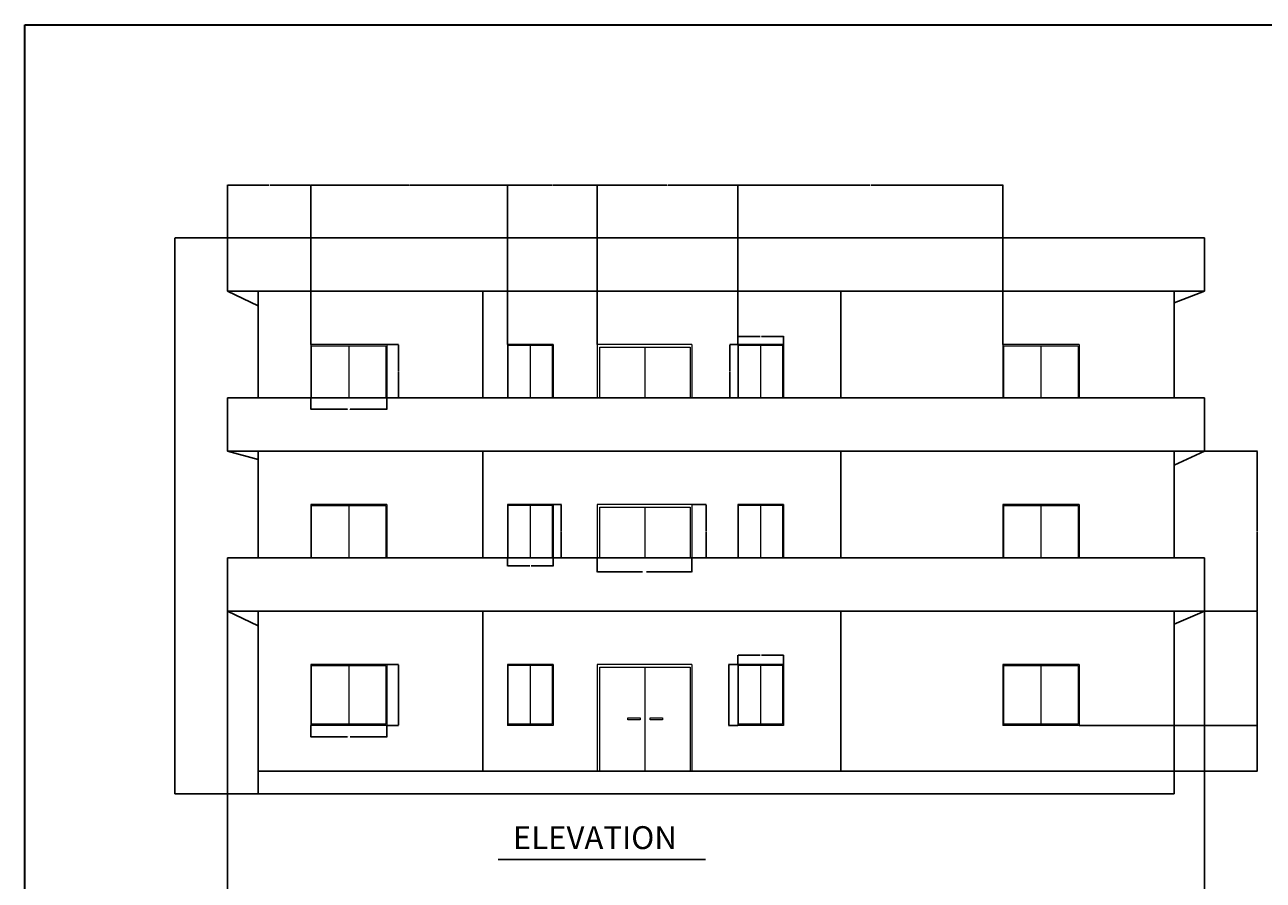
# Model space of a CAD drawing. Units: inches. Extents: x 2185 to 4426, y 1138 to 3073.
# Tile 7 of 14: x 2185 to 3160, y 2400 to 3073. Entities that reach past the tile are written whole.
import ezdxf

# ---------------------------------------------------------------- set-up
doc = ezdxf.new("R2010")
doc.units = ezdxf.units.IN
for name, color, linetype, lineweight in [('A-ANNO-DIMS', 2, 'Continuous', 18), ('A-ANNO-TITL', 7, 'Continuous', 25), ('A-ANNO-TTLB', 7, 'Continuous', 35), ('A-ELEV', 7, 'Continuous', 25), ('A-ELEV-DOOR', 3, 'Continuous', 18), ('A-ELEV-GLAZ', 4, 'Continuous', 18)]:
    doc.layers.add(name, color=color, linetype=linetype, lineweight=lineweight)
doc.styles.get("Standard").update_dxf_attribs({"font": 'arial.ttf'})
doc.dimstyles.get("Standard").update_dxf_attribs({"dimtxt": 0.18, "dimasz": 0.18, "dimexe": 0.18, "dimexo": 0.0625, "dimgap": 0.09, "dimtad": 0, "dimtih": 1, "dimtoh": 1, "dimdec": 4, "dimzin": 0, "dimdsep": 46, "dimtxsty": 'Standard', "dimcen": 0.09, "dimadec": 0, "dimazin": 0, "dimtfac": 1, "dimtdec": 4, "dimtofl": 0, "dimtmove": 0, "dimatfit": 3, "dimfxl": 1, "dimtolj": 1, "dimtzin": 0, "dimarcsym": 0})

# ---------------------------------------------------------------- blocks, each defined once
blk = doc.blocks.new('WIN-ELEV-WIDE-LOWER')
for p, q in [((0, 48), (0, 0)), ((60, 48), (0, 48)), ((0, 48), (0, 0)), ((60, 48), (0, 48)), ((29.88, 47.09), (29.88, 0.99)), ((60, 48), (60, 0)), ((60, 48), (60, 0)), ((60, 0), (0, 0)), ((60, 0), (0, 0))]:
    blk.add_line(p, q)
blk.add_lwpolyline([(0.58, 47.09), (59.17, 47.09), (59.17, 0.99), (0.58, 0.99)], close=True)
blk = doc.blocks.new('WIN-ELEV-WIDE-UPPER')
for p, q in [((0, 42), (0, 0)), ((60, 42), (0, 42)), ((0, 42), (0, 0)), ((60, 42), (0, 42)), ((29.88, 41.09), (29.88, 0)), ((60, 42), (60, 0)), ((60, 42), (60, 0))]:
    blk.add_line(p, q)
blk.add_lwpolyline([(0.58, 0), (0.58, 41.09), (59.17, 41.09), (59.17, 0)])
blk = doc.blocks.new('WIN-ELEV-NARROW-UPPER')
for p, q in [((0, 42), (0, 0)), ((36, 42), (0, 42)), ((0, 42), (0, 0)), ((36, 42), (0, 42)), ((0, 42), (0, 0)), ((17.83, 41.41), (17.83, 0)), ((36, 42), (36, 0)), ((36, 42), (36, 0)), ((36, 42), (36, 0))]:
    blk.add_line(p, q)
blk.add_lwpolyline([(0.51, 0), (0.51, 41.41), (35.15, 41.41), (35.15, 0)])
blk = doc.blocks.new('WIN-ELEV-NARROW-LOWER-TYPE-B')
for p, q in [((0, 48), (0, 0)), ((36, 48), (0, 48)), ((17.83, 47.41), (17.83, 0.85)), ((36, 48), (36, 0)), ((36, 0), (0, 0))]:
    blk.add_line(p, q)
blk.add_lwpolyline([(0.51, 47.41), (35.15, 47.41), (35.15, 0.85), (0.51, 0.85)], close=True)
blk = doc.blocks.new('WIN-ELEV-NARROW-UPPER-TYPE-B')
for p, q in [((0, 42), (0, 0)), ((36, 42), (0, 42)), ((17.83, 41.41), (17.83, 0)), ((36, 42), (36, 0))]:
    blk.add_line(p, q)
blk.add_lwpolyline([(0.51, 0), (0.51, 41.41), (35.15, 41.41), (35.15, 0)])
blk = doc.blocks.new('DOOR-ELEV-DOUBLE-UPPER-TYPE-B')
for p, q in [((0, 42), (0, 0)), ((74.51, 42), (0, 42)), ((37.6, 39.93), (37.6, 0)), ((74.51, 42), (74.51, 0))]:
    blk.add_line(p, q)
blk.add_lwpolyline([(2.14, 0), (2.14, 39.93), (73.06, 39.93), (73.06, 0)])
blk = doc.blocks.new('*D126')
at = {"layer": 'A-ANNO-DIMS', "color": 0, "lineweight": -2, "transparency": 16777216}
for p, q in [((2410.04, 2521.42), (2410.04, 2512.3)), ((2470.04, 2521.42), (2470.04, 2512.3)), ((2410.22, 2512.48), (2438.92, 2512.48)), ((2469.86, 2512.48), (2441.16, 2512.48))]:
    blk.add_line(p, q, dxfattribs=at)
at = {"layer": 'A-ANNO-DIMS', "color": 0, "transparency": 16777216}
for points in [[(2410.22, 2512.51), (2410.22, 2512.45), (2410.04, 2512.48)], [(2469.86, 2512.51), (2469.86, 2512.45), (2470.04, 2512.48)]]:
    blk.add_solid(points, dxfattribs=at)
at = {"layer": 'Defpoints', "color": 0, "transparency": 16777216}
for p in [(2410.04, 2521.48), (2470.04, 2521.48), (2470.04, 2512.48)]:
    blk.add_point(p, dxfattribs=at)
at = {"layer": 'A-ANNO-DIMS', "color": 0, "transparency": 16777216, "insert": (2440.04, 2512.48), "char_height": 0.18, "attachment_point": 5}
blk.add_mtext('\\A1;WINDOW 60 TYP.', dxfattribs=at)
blk = doc.blocks.new('*D127')
at = {"layer": 'A-ANNO-DIMS', "color": 0, "lineweight": -2, "transparency": 16777216}
for p, q in [((2470.1, 2569.48), (2479.22, 2569.48)), ((2479.04, 2569.3), (2479.04, 2545.66)), ((2479.04, 2521.66), (2479.04, 2545.3)), ((2470.1, 2521.48), (2479.22, 2521.48))]:
    blk.add_line(p, q, dxfattribs=at)
at = {"layer": 'A-ANNO-DIMS', "color": 0, "transparency": 16777216}
for points in [[(2479.01, 2569.3), (2479.07, 2569.3), (2479.04, 2569.48)], [(2479.01, 2521.66), (2479.07, 2521.66), (2479.04, 2521.48)]]:
    blk.add_solid(points, dxfattribs=at)
at = {"layer": 'Defpoints', "color": 0, "transparency": 16777216}
for p in [(2470.04, 2569.48), (2479.04, 2569.48), (2470.04, 2521.48)]:
    blk.add_point(p, dxfattribs=at)
at = {"layer": 'A-ANNO-DIMS', "color": 0, "transparency": 16777216, "insert": (2479.04, 2545.48), "char_height": 0.18, "attachment_point": 5}
blk.add_mtext('\\A1;48 TYP.', dxfattribs=at)
blk = doc.blocks.new('*D128')
at = {"layer": 'A-ANNO-DIMS', "color": 0, "lineweight": -2, "transparency": 16777216}
for p, q in [((2410.04, 2779.42), (2410.04, 2770.3)), ((2410.22, 2770.48), (2438.92, 2770.48)), ((2469.86, 2770.48), (2441.16, 2770.48)), ((2470.04, 2779.42), (2470.04, 2770.3))]:
    blk.add_line(p, q, dxfattribs=at)
at = {"layer": 'A-ANNO-DIMS', "color": 0, "transparency": 16777216}
for points in [[(2410.22, 2770.51), (2410.22, 2770.45), (2410.04, 2770.48)], [(2469.86, 2770.51), (2469.86, 2770.45), (2470.04, 2770.48)]]:
    blk.add_solid(points, dxfattribs=at)
at = {"layer": 'Defpoints', "color": 0, "transparency": 16777216}
for p in [(2410.04, 2779.48), (2470.04, 2779.48), (2470.04, 2770.48)]:
    blk.add_point(p, dxfattribs=at)
at = {"layer": 'A-ANNO-DIMS', "color": 0, "transparency": 16777216, "insert": (2440.04, 2770.48), "char_height": 0.18, "attachment_point": 5}
blk.add_mtext('\\A1;WINDOW 60 TYP.', dxfattribs=at)
blk = doc.blocks.new('*D129')
at = {"layer": 'A-ANNO-DIMS', "color": 0, "lineweight": -2, "transparency": 16777216}
for p, q in [((2470.1, 2821.48), (2479.22, 2821.48)), ((2479.04, 2821.3), (2479.04, 2800.66)), ((2479.04, 2779.66), (2479.04, 2800.3)), ((2470.1, 2779.48), (2479.22, 2779.48))]:
    blk.add_line(p, q, dxfattribs=at)
at = {"layer": 'A-ANNO-DIMS', "color": 0, "transparency": 16777216}
for points in [[(2479.01, 2821.3), (2479.07, 2821.3), (2479.04, 2821.48)], [(2479.01, 2779.66), (2479.07, 2779.66), (2479.04, 2779.48)]]:
    blk.add_solid(points, dxfattribs=at)
at = {"layer": 'Defpoints', "color": 0, "transparency": 16777216}
for p in [(2470.04, 2821.48), (2479.04, 2821.48), (2470.04, 2779.48)]:
    blk.add_point(p, dxfattribs=at)
at = {"layer": 'A-ANNO-DIMS', "color": 0, "transparency": 16777216, "insert": (2479.04, 2800.48), "char_height": 0.18, "attachment_point": 5}
blk.add_mtext('\\A1;42 TYP.', dxfattribs=at)
blk = doc.blocks.new('*D130')
at = {"layer": 'A-ANNO-DIMS', "color": 0, "lineweight": -2, "transparency": 16777216}
for p, q in [((2601.1, 2695.48), (2607.52, 2695.48)), ((2607.34, 2695.3), (2607.34, 2674.67)), ((2607.34, 2653.66), (2607.34, 2674.3)), ((2601.1, 2653.48), (2607.52, 2653.48))]:
    blk.add_line(p, q, dxfattribs=at)
at = {"layer": 'A-ANNO-DIMS', "color": 0, "transparency": 16777216}
for points in [[(2607.31, 2695.3), (2607.37, 2695.3), (2607.34, 2695.48)], [(2607.31, 2653.66), (2607.37, 2653.66), (2607.34, 2653.48)]]:
    blk.add_solid(points, dxfattribs=at)
at = {"layer": 'Defpoints', "color": 0, "transparency": 16777216}
for p in [(2601.04, 2695.48), (2607.34, 2695.48), (2601.04, 2653.48)]:
    blk.add_point(p, dxfattribs=at)
at = {"layer": 'A-ANNO-DIMS', "color": 0, "transparency": 16777216, "insert": (2607.34, 2674.48), "char_height": 0.18, "attachment_point": 5}
blk.add_mtext('\\A1;SASH 42 TYP.', dxfattribs=at)
blk = doc.blocks.new('*D131')
at = {"layer": 'A-ANNO-DIMS', "color": 0, "lineweight": -2, "transparency": 16777216}
for p, q in [((2565.04, 2653.42), (2565.04, 2647)), ((2601.04, 2653.42), (2601.04, 2647)), ((2565.22, 2647.18), (2582.51, 2647.18)), ((2600.86, 2647.18), (2583.57, 2647.18))]:
    blk.add_line(p, q, dxfattribs=at)
at = {"layer": 'A-ANNO-DIMS', "color": 0, "transparency": 16777216}
for points in [[(2565.22, 2647.21), (2565.22, 2647.15), (2565.04, 2647.18)], [(2600.86, 2647.21), (2600.86, 2647.15), (2601.04, 2647.18)]]:
    blk.add_solid(points, dxfattribs=at)
at = {"layer": 'Defpoints', "color": 0, "transparency": 16777216}
for p in [(2565.04, 2653.48), (2601.04, 2653.48), (2601.04, 2647.18)]:
    blk.add_point(p, dxfattribs=at)
at = {"layer": 'A-ANNO-DIMS', "color": 0, "transparency": 16777216, "insert": (2583.04, 2647.18), "char_height": 0.18, "attachment_point": 5}
blk.add_mtext('\\A1;36 TYP.', dxfattribs=at)
blk = doc.blocks.new('*D132')
at = {"layer": 'A-ANNO-DIMS', "color": 0, "lineweight": -2, "transparency": 16777216}
for p, q in [((2746.37, 2569.48), (2739.05, 2569.48)), ((2739.23, 2569.3), (2739.23, 2545.67)), ((2739.23, 2521.66), (2739.23, 2545.3)), ((2746.37, 2521.48), (2739.05, 2521.48))]:
    blk.add_line(p, q, dxfattribs=at)
at = {"layer": 'A-ANNO-DIMS', "color": 0, "transparency": 16777216}
for points in [[(2739.2, 2569.3), (2739.26, 2569.3), (2739.23, 2569.48)], [(2739.2, 2521.66), (2739.26, 2521.66), (2739.23, 2521.48)]]:
    blk.add_solid(points, dxfattribs=at)
at = {"layer": 'Defpoints', "color": 0, "transparency": 16777216}
for p in [(2739.23, 2569.48), (2746.43, 2569.48), (2746.43, 2521.48)]:
    blk.add_point(p, dxfattribs=at)
at = {"layer": 'A-ANNO-DIMS', "color": 0, "transparency": 16777216, "insert": (2739.23, 2545.48), "char_height": 0.18, "attachment_point": 5}
blk.add_mtext('\\A1;SASH 48 TYP.', dxfattribs=at)
blk = doc.blocks.new('*D133')
at = {"layer": 'A-ANNO-DIMS', "color": 0, "lineweight": -2, "transparency": 16777216}
for p, q in [((2746.43, 2569.54), (2746.43, 2576.86)), ((2746.61, 2576.68), (2763.9, 2576.68)), ((2782.25, 2576.68), (2764.96, 2576.68)), ((2782.43, 2569.54), (2782.43, 2576.86))]:
    blk.add_line(p, q, dxfattribs=at)
at = {"layer": 'A-ANNO-DIMS', "color": 0, "transparency": 16777216}
for points in [[(2746.61, 2576.71), (2746.61, 2576.65), (2746.43, 2576.68)], [(2782.25, 2576.71), (2782.25, 2576.65), (2782.43, 2576.68)]]:
    blk.add_solid(points, dxfattribs=at)
at = {"layer": 'Defpoints', "color": 0, "transparency": 16777216}
for p in [(2782.43, 2576.68), (2746.43, 2569.48), (2782.43, 2569.48)]:
    blk.add_point(p, dxfattribs=at)
at = {"layer": 'A-ANNO-DIMS', "color": 0, "transparency": 16777216, "insert": (2764.43, 2576.68), "char_height": 0.18, "attachment_point": 5}
blk.add_mtext('\\A1;36 TYP.', dxfattribs=at)
blk = doc.blocks.new('*D134')
at = {"layer": 'A-ANNO-DIMS', "color": 0, "lineweight": -2, "transparency": 16777216}
for p, q in [((2746.37, 2821.48), (2739.95, 2821.48)), ((2740.13, 2821.3), (2740.13, 2800.67)), ((2740.13, 2779.66), (2740.13, 2800.3)), ((2746.37, 2779.48), (2739.95, 2779.48))]:
    blk.add_line(p, q, dxfattribs=at)
at = {"layer": 'A-ANNO-DIMS', "color": 0, "transparency": 16777216}
for points in [[(2740.1, 2821.3), (2740.16, 2821.3), (2740.13, 2821.48)], [(2740.1, 2779.66), (2740.16, 2779.66), (2740.13, 2779.48)]]:
    blk.add_solid(points, dxfattribs=at)
at = {"layer": 'Defpoints', "color": 0, "transparency": 16777216}
for p in [(2740.13, 2821.48), (2746.43, 2821.48), (2746.43, 2779.48)]:
    blk.add_point(p, dxfattribs=at)
at = {"layer": 'A-ANNO-DIMS', "color": 0, "transparency": 16777216, "insert": (2740.13, 2800.48), "char_height": 0.18, "attachment_point": 5}
blk.add_mtext('\\A1;SASH 42 TYP.', dxfattribs=at)
blk = doc.blocks.new('*D135')
at = {"layer": 'A-ANNO-DIMS', "color": 0, "lineweight": -2, "transparency": 16777216}
for p, q in [((2746.43, 2821.54), (2746.43, 2827.96)), ((2746.61, 2827.78), (2763.9, 2827.78)), ((2782.25, 2827.78), (2764.96, 2827.78)), ((2782.43, 2821.54), (2782.43, 2827.96))]:
    blk.add_line(p, q, dxfattribs=at)
at = {"layer": 'A-ANNO-DIMS', "color": 0, "transparency": 16777216}
for points in [[(2746.61, 2827.81), (2746.61, 2827.75), (2746.43, 2827.78)], [(2782.25, 2827.81), (2782.25, 2827.75), (2782.43, 2827.78)]]:
    blk.add_solid(points, dxfattribs=at)
at = {"layer": 'Defpoints', "color": 0, "transparency": 16777216}
for p in [(2746.43, 2821.48), (2782.43, 2827.78), (2782.43, 2821.48)]:
    blk.add_point(p, dxfattribs=at)
at = {"layer": 'A-ANNO-DIMS', "color": 0, "transparency": 16777216, "insert": (2764.43, 2827.78), "char_height": 0.18, "attachment_point": 5}
blk.add_mtext('\\A1;36 TYP.', dxfattribs=at)
blk = doc.blocks.new('*D136')
at = {"layer": 'A-ANNO-DIMS', "color": 0, "lineweight": -2, "transparency": 16777216}
for p, q in [((2635.64, 2653.42), (2635.64, 2642.13)), ((2710.16, 2653.42), (2710.16, 2642.13)), ((2635.82, 2642.31), (2671.38, 2642.31)), ((2709.98, 2642.31), (2674.42, 2642.31))]:
    blk.add_line(p, q, dxfattribs=at)
at = {"layer": 'A-ANNO-DIMS', "color": 0, "transparency": 16777216}
for points in [[(2635.82, 2642.34), (2635.82, 2642.28), (2635.64, 2642.31)], [(2709.98, 2642.34), (2709.98, 2642.28), (2710.16, 2642.31)]]:
    blk.add_solid(points, dxfattribs=at)
at = {"layer": 'Defpoints', "color": 0, "transparency": 16777216}
for p in [(2635.64, 2653.48), (2710.16, 2653.48), (2710.16, 2642.31)]:
    blk.add_point(p, dxfattribs=at)
at = {"layer": 'A-ANNO-DIMS', "color": 0, "transparency": 16777216, "insert": (2672.9, 2642.31), "char_height": 0.18, "attachment_point": 5}
blk.add_mtext('\\A1;PAIRED DOORS 75 TYP.', dxfattribs=at)
blk = doc.blocks.new('*D137')
at = {"layer": 'A-ANNO-DIMS', "color": 0, "lineweight": -2, "transparency": 16777216}
for p, q in [((2710.22, 2695.48), (2721.51, 2695.48)), ((2721.33, 2695.3), (2721.33, 2674.66)), ((2721.33, 2653.66), (2721.33, 2674.3)), ((2710.22, 2653.48), (2721.51, 2653.48))]:
    blk.add_line(p, q, dxfattribs=at)
at = {"layer": 'A-ANNO-DIMS', "color": 0, "transparency": 16777216}
for points in [[(2721.3, 2695.3), (2721.36, 2695.3), (2721.33, 2695.48)], [(2721.3, 2653.66), (2721.36, 2653.66), (2721.33, 2653.48)]]:
    blk.add_solid(points, dxfattribs=at)
at = {"layer": 'Defpoints', "color": 0, "transparency": 16777216}
for p in [(2710.16, 2695.48), (2721.33, 2695.48), (2710.16, 2653.48)]:
    blk.add_point(p, dxfattribs=at)
at = {"layer": 'A-ANNO-DIMS', "color": 0, "transparency": 16777216, "insert": (2721.33, 2674.48), "char_height": 0.18, "attachment_point": 5}
blk.add_mtext('\\A1;42 TYP.', dxfattribs=at)
blk = doc.blocks.new('*D162')
at = {"layer": 'A-ANNO-DIMS', "color": 0, "lineweight": -2, "transparency": 16777216}
for p, q in [((2344.52, 2611.42), (2344.52, 2374.27)), ((3114.02, 2611.42), (3114.02, 2374.27)), ((2344.7, 2374.45), (2728.88, 2374.45)), ((3113.84, 2374.45), (2729.66, 2374.45))]:
    blk.add_line(p, q, dxfattribs=at)
at = {"layer": 'A-ANNO-DIMS', "color": 0, "transparency": 16777216}
for points in [[(2344.7, 2374.48), (2344.7, 2374.42), (2344.52, 2374.45)], [(3113.84, 2374.48), (3113.84, 2374.42), (3114.02, 2374.45)]]:
    blk.add_solid(points, dxfattribs=at)
at = {"layer": 'Defpoints', "color": 0, "transparency": 16777216}
for p in [(2344.52, 2611.48), (3114.02, 2611.48), (3114.02, 2374.45)]:
    blk.add_point(p, dxfattribs=at)
at = {"layer": 'A-ANNO-DIMS', "color": 0, "transparency": 16777216, "insert": (2729.27, 2374.45), "char_height": 0.18, "attachment_point": 5}
blk.add_mtext('\\A1;769.5', dxfattribs=at)
blk = doc.blocks.new('*D163')
at = {"layer": 'A-ANNO-DIMS', "color": 0, "lineweight": -2, "transparency": 16777216}
for p, q in [((2344.46, 2905.48), (2302.84, 2905.48)), ((2303.02, 2905.3), (2303.02, 2686.66)), ((2303.02, 2467.66), (2303.02, 2686.3)), ((2368.46, 2467.48), (2302.84, 2467.48))]:
    blk.add_line(p, q, dxfattribs=at)
at = {"layer": 'A-ANNO-DIMS', "color": 0, "transparency": 16777216}
for points in [[(2302.99, 2905.3), (2303.05, 2905.3), (2303.02, 2905.48)], [(2302.99, 2467.66), (2303.05, 2467.66), (2303.02, 2467.48)]]:
    blk.add_solid(points, dxfattribs=at)
at = {"layer": 'Defpoints', "color": 0, "transparency": 16777216}
for p in [(2303.02, 2905.48), (2344.52, 2905.48), (2368.52, 2467.48)]:
    blk.add_point(p, dxfattribs=at)
at = {"layer": 'A-ANNO-DIMS', "color": 0, "transparency": 16777216, "insert": (2303.02, 2686.48), "char_height": 0.18, "attachment_point": 5}
blk.add_mtext('\\A1;438', dxfattribs=at)
blk = doc.blocks.new('*D164')
at = {"layer": 'A-ANNO-DIMS', "color": 0, "lineweight": -2, "transparency": 16777216}
for p, q in [((2344.52, 2905.54), (2344.52, 2947.16)), ((2344.7, 2946.98), (2376.89, 2946.98)), ((2409.86, 2946.98), (2377.67, 2946.98)), ((2410.04, 2821.54), (2410.04, 2947.16))]:
    blk.add_line(p, q, dxfattribs=at)
at = {"layer": 'A-ANNO-DIMS', "color": 0, "transparency": 16777216}
for points in [[(2344.7, 2947.01), (2344.7, 2946.95), (2344.52, 2946.98)], [(2409.86, 2947.01), (2409.86, 2946.95), (2410.04, 2946.98)]]:
    blk.add_solid(points, dxfattribs=at)
at = {"layer": 'Defpoints', "color": 0, "transparency": 16777216}
for p in [(2410.04, 2946.98), (2344.52, 2905.48), (2410.04, 2821.48)]:
    blk.add_point(p, dxfattribs=at)
at = {"layer": 'A-ANNO-DIMS', "color": 0, "transparency": 16777216, "insert": (2377.28, 2946.98), "char_height": 0.18, "attachment_point": 5}
blk.add_mtext('\\A1;65.52', dxfattribs=at)
blk = doc.blocks.new('*D165')
at = {"layer": 'A-ANNO-DIMS', "color": 0, "lineweight": -2, "transparency": 16777216}
for p, q in [((2410.04, 2821.54), (2410.04, 2947.16)), ((2410.22, 2946.98), (2487.26, 2946.98)), ((2564.86, 2946.98), (2487.82, 2946.98)), ((2565.04, 2821.54), (2565.04, 2947.16))]:
    blk.add_line(p, q, dxfattribs=at)
at = {"layer": 'A-ANNO-DIMS', "color": 0, "transparency": 16777216}
for points in [[(2410.22, 2947.01), (2410.22, 2946.95), (2410.04, 2946.98)], [(2564.86, 2947.01), (2564.86, 2946.95), (2565.04, 2946.98)]]:
    blk.add_solid(points, dxfattribs=at)
at = {"layer": 'Defpoints', "color": 0, "transparency": 16777216}
for p in [(2565.04, 2946.98), (2410.04, 2821.48), (2565.04, 2821.48)]:
    blk.add_point(p, dxfattribs=at)
at = {"layer": 'A-ANNO-DIMS', "color": 0, "transparency": 16777216, "insert": (2487.54, 2946.98), "char_height": 0.18, "attachment_point": 5}
blk.add_mtext('\\A1;155', dxfattribs=at)
blk = doc.blocks.new('*D166')
at = {"layer": 'A-ANNO-DIMS', "color": 0, "lineweight": -2, "transparency": 16777216}
for p, q in [((2565.04, 2821.54), (2565.04, 2947.16)), ((2565.22, 2946.98), (2600.02, 2946.98)), ((2635.46, 2946.98), (2600.66, 2946.98)), ((2635.64, 2821.54), (2635.64, 2947.16))]:
    blk.add_line(p, q, dxfattribs=at)
at = {"layer": 'A-ANNO-DIMS', "color": 0, "transparency": 16777216}
for points in [[(2565.22, 2947.01), (2565.22, 2946.95), (2565.04, 2946.98)], [(2635.46, 2947.01), (2635.46, 2946.95), (2635.64, 2946.98)]]:
    blk.add_solid(points, dxfattribs=at)
at = {"layer": 'Defpoints', "color": 0, "transparency": 16777216}
for p in [(2635.64, 2946.98), (2565.04, 2821.48), (2635.64, 2821.48)]:
    blk.add_point(p, dxfattribs=at)
at = {"layer": 'A-ANNO-DIMS', "color": 0, "transparency": 16777216, "insert": (2600.34, 2946.98), "char_height": 0.18, "attachment_point": 5}
blk.add_mtext('\\A1;70.6', dxfattribs=at)
blk = doc.blocks.new('*D167')
at = {"layer": 'A-ANNO-DIMS', "color": 0, "lineweight": -2, "transparency": 16777216}
for p, q in [((2635.64, 2821.54), (2635.64, 2947.16)), ((2635.82, 2946.98), (2690.58, 2946.98)), ((2746.25, 2946.98), (2691.49, 2946.98)), ((2746.43, 2821.54), (2746.43, 2947.16))]:
    blk.add_line(p, q, dxfattribs=at)
at = {"layer": 'A-ANNO-DIMS', "color": 0, "transparency": 16777216}
for points in [[(2635.82, 2947.01), (2635.82, 2946.95), (2635.64, 2946.98)], [(2746.25, 2947.01), (2746.25, 2946.95), (2746.43, 2946.98)]]:
    blk.add_solid(points, dxfattribs=at)
at = {"layer": 'Defpoints', "color": 0, "transparency": 16777216}
for p in [(2746.43, 2946.98), (2635.64, 2821.48), (2746.43, 2821.48)]:
    blk.add_point(p, dxfattribs=at)
at = {"layer": 'A-ANNO-DIMS', "color": 0, "transparency": 16777216, "insert": (2691.04, 2946.98), "char_height": 0.18, "attachment_point": 5}
blk.add_mtext('\\A1;110.79', dxfattribs=at)
blk = doc.blocks.new('*D168')
at = {"layer": 'A-ANNO-DIMS', "color": 0, "lineweight": -2, "transparency": 16777216}
for p, q in [((2746.43, 2821.54), (2746.43, 2947.16)), ((2746.61, 2946.98), (2850.43, 2946.98)), ((2955.03, 2946.98), (2851.22, 2946.98)), ((2955.21, 2821.54), (2955.21, 2947.16))]:
    blk.add_line(p, q, dxfattribs=at)
at = {"layer": 'A-ANNO-DIMS', "color": 0, "transparency": 16777216}
for points in [[(2746.61, 2947.01), (2746.61, 2946.95), (2746.43, 2946.98)], [(2955.03, 2947.01), (2955.03, 2946.95), (2955.21, 2946.98)]]:
    blk.add_solid(points, dxfattribs=at)
at = {"layer": 'Defpoints', "color": 0, "transparency": 16777216}
for p in [(2955.21, 2946.98), (2746.43, 2821.48), (2955.21, 2821.48)]:
    blk.add_point(p, dxfattribs=at)
at = {"layer": 'A-ANNO-DIMS', "color": 0, "transparency": 16777216, "insert": (2850.82, 2946.98), "char_height": 0.18, "attachment_point": 5}
blk.add_mtext('\\A1;208.8', dxfattribs=at)
blk = doc.blocks.new('*D169')
at = {"layer": 'A-ANNO-DIMS', "color": 0, "lineweight": -2, "transparency": 16777216}
for p, q in [((3015.27, 2521.48), (3155.7, 2521.48)), ((3155.52, 2521.3), (3155.52, 2503.66)), ((3155.52, 2485.66), (3155.52, 2503.3)), ((3090.08, 2485.48), (3155.7, 2485.48))]:
    blk.add_line(p, q, dxfattribs=at)
at = {"layer": 'A-ANNO-DIMS', "color": 0, "transparency": 16777216}
for points in [[(3155.49, 2521.3), (3155.55, 2521.3), (3155.52, 2521.48)], [(3155.49, 2485.66), (3155.55, 2485.66), (3155.52, 2485.48)]]:
    blk.add_solid(points, dxfattribs=at)
at = {"layer": 'Defpoints', "color": 0, "transparency": 16777216}
for p in [(3015.21, 2521.48), (3155.52, 2521.48), (3090.02, 2485.48)]:
    blk.add_point(p, dxfattribs=at)
at = {"layer": 'A-ANNO-DIMS', "color": 0, "transparency": 16777216, "insert": (3155.52, 2503.48), "char_height": 0.18, "attachment_point": 5}
blk.add_mtext('\\A1;36', dxfattribs=at)
blk = doc.blocks.new('*D170')
at = {"layer": 'A-ANNO-DIMS', "color": 0, "lineweight": -2, "transparency": 16777216}
for p, q in [((3114.08, 2611.48), (3155.7, 2611.48)), ((3155.52, 2611.3), (3155.52, 2566.66)), ((3155.52, 2521.66), (3155.52, 2566.3)), ((3015.27, 2521.48), (3155.7, 2521.48))]:
    blk.add_line(p, q, dxfattribs=at)
at = {"layer": 'A-ANNO-DIMS', "color": 0, "transparency": 16777216}
for points in [[(3155.49, 2611.3), (3155.55, 2611.3), (3155.52, 2611.48)], [(3155.49, 2521.66), (3155.55, 2521.66), (3155.52, 2521.48)]]:
    blk.add_solid(points, dxfattribs=at)
at = {"layer": 'Defpoints', "color": 0, "transparency": 16777216}
for p in [(3114.02, 2611.48), (3155.52, 2611.48), (3015.21, 2521.48)]:
    blk.add_point(p, dxfattribs=at)
at = {"layer": 'A-ANNO-DIMS', "color": 0, "transparency": 16777216, "insert": (3155.52, 2566.48), "char_height": 0.18, "attachment_point": 5}
blk.add_mtext('\\A1;90', dxfattribs=at)
blk = doc.blocks.new('*D171')
at = {"layer": 'A-ANNO-DIMS', "color": 0, "lineweight": -2, "transparency": 16777216}
for p, q in [((3114.08, 2737.48), (3155.7, 2737.48)), ((3155.52, 2737.3), (3155.52, 2674.66)), ((3155.52, 2611.66), (3155.52, 2674.3)), ((3114.08, 2611.48), (3155.7, 2611.48))]:
    blk.add_line(p, q, dxfattribs=at)
at = {"layer": 'A-ANNO-DIMS', "color": 0, "transparency": 16777216}
for points in [[(3155.49, 2737.3), (3155.55, 2737.3), (3155.52, 2737.48)], [(3155.49, 2611.66), (3155.55, 2611.66), (3155.52, 2611.48)]]:
    blk.add_solid(points, dxfattribs=at)
at = {"layer": 'Defpoints', "color": 0, "transparency": 16777216}
for p in [(3114.02, 2737.48), (3155.52, 2737.48), (3114.02, 2611.48)]:
    blk.add_point(p, dxfattribs=at)
at = {"layer": 'A-ANNO-DIMS', "color": 0, "transparency": 16777216, "insert": (3155.52, 2674.48), "char_height": 0.18, "attachment_point": 5}
blk.add_mtext('\\A1;126', dxfattribs=at)

msp = doc.modelspace()

# ---------------------------------------------------------------- linework, layer by layer
at = {"layer": 'A-ANNO-TITL'}
msp.add_line((2557.491, 2415.951), (2720.974, 2415.951), dxfattribs=at)
at = {"layer": 'A-ANNO-TTLB'}
msp.add_lwpolyline([(2184.741, 3073.364), (4426.252, 3073.364), (4426.252, 1137.99), (2184.741, 1137.99)], close=True, dxfattribs=at)
at = {"layer": 'A-ELEV'}
for p, q in [((3114.019, 2905.482), (2344.519, 2905.482)), ((2344.519, 2863.482), (2344.519, 2905.482)), ((3114.019, 2863.482), (3114.019, 2905.482)), ((3114.019, 2863.482), (2344.519, 2863.482)), ((2344.519, 2863.482), (2368.519, 2852.046)), ((2368.519, 2863.482), (2368.519, 2779.482)), ((2545.519, 2863.482), (2545.519, 2779.482)), ((2827.519, 2863.482), (2827.519, 2779.482)), ((3090.019, 2863.482), (3090.019, 2779.482)), ((3114.019, 2863.482), (3090.019, 2854.345)), ((3114.019, 2779.482), (2344.519, 2779.482)), ((2344.519, 2737.482), (2344.519, 2779.482)), ((3114.019, 2737.482), (3114.019, 2779.482)), ((3114.019, 2737.482), (2344.519, 2737.482)), ((2344.519, 2737.482), (2368.519, 2730.937)), ((2368.519, 2737.482), (2368.519, 2653.482)), ((2368.519, 2737.482), (2368.519, 2719.482)), ((2545.519, 2737.482), (2545.519, 2653.482)), ((2827.519, 2737.482), (2827.519, 2653.482)), ((3090.019, 2653.482), (3090.019, 2737.482)), ((3114.019, 2737.482), (3090.019, 2726.494)), ((3114.019, 2653.482), (2344.519, 2653.482)), ((2344.519, 2611.482), (2344.519, 2653.482)), ((3114.019, 2611.482), (3114.019, 2653.482)), ((3114.019, 2611.482), (2344.519, 2611.482)), ((2344.519, 2611.482), (2368.519, 2599.913)), ((2368.519, 2611.482), (2368.519, 2467.482)), ((2368.519, 2611.482), (2368.519, 2593.482)), ((2545.519, 2611.482), (2545.519, 2485.482)), ((2827.519, 2611.482), (2827.519, 2485.482)), ((3090.019, 2611.482), (3090.019, 2467.482)), ((3114.019, 2611.482), (3090.019, 2601.195)), ((3090.019, 2485.482), (2368.519, 2485.482)), ((3090.019, 2467.482), (2368.519, 2467.482))]:
    msp.add_line(p, q, dxfattribs=at)
at = {"layer": 'A-ELEV-DOOR'}
for p, q in [((2635.644, 2821.482), (2635.644, 2779.482)), ((2710.156, 2821.482), (2635.644, 2821.482)), ((2635.644, 2821.482), (2635.644, 2779.482)), ((2710.156, 2821.482), (2635.644, 2821.482)), ((2673.245, 2819.417), (2673.245, 2779.482)), ((2710.156, 2821.482), (2710.156, 2779.482)), ((2710.156, 2821.482), (2710.156, 2779.482)), ((2635.644, 2695.482), (2635.644, 2653.482)), ((2710.156, 2695.482), (2635.644, 2695.482)), ((2710.156, 2695.482), (2710.156, 2653.482)), ((2635.644, 2569.482), (2635.644, 2485.482)), ((2710.156, 2569.482), (2635.644, 2569.482)), ((2673.245, 2567.417), (2673.245, 2485.482)), ((2710.156, 2569.482), (2710.156, 2485.482))]:
    msp.add_line(p, q, dxfattribs=at)
for points in [[(2637.783, 2779.482), (2637.783, 2819.417), (2708.706, 2819.417), (2708.706, 2779.482)], [(2708.706, 2737.482), (2708.706, 2737.482), (2637.783, 2737.482)], [(2708.706, 2737.482), (2708.706, 2737.482), (2637.783, 2737.482)], [(2708.706, 2611.482), (2637.783, 2611.482)]]:
    msp.add_lwpolyline(points, dxfattribs=at)
for points in [[(2637.783, 2567.417), (2708.706, 2567.417), (2708.706, 2485.482), (2637.783, 2485.482)], [(2659.678, 2527.551), (2669.475, 2527.551), (2669.475, 2525.734), (2659.678, 2525.734)], [(2677.287, 2527.551), (2687.083, 2527.551), (2687.083, 2525.734), (2677.287, 2525.734)]]:
    msp.add_lwpolyline(points, close=True, dxfattribs=at)
at = {"layer": 'A-ELEV-GLAZ'}
for p, q in [((2955.211, 2821.482), (2955.211, 2779.482)), ((3015.211, 2821.482), (2955.211, 2821.482)), ((2985.088, 2820.575), (2985.088, 2779.482)), ((3015.211, 2821.482), (3015.211, 2779.482)), ((2746.431, 2695.482), (2746.431, 2653.482)), ((2782.431, 2695.482), (2782.431, 2653.482)), ((2955.211, 2695.482), (2955.211, 2653.482)), ((3015.211, 2695.482), (2955.211, 2695.482)), ((2955.211, 2695.482), (2955.211, 2653.482)), ((3015.211, 2695.482), (2955.211, 2695.482)), ((2985.211, 2653.482), (2985.211, 2694.575)), ((3015.211, 2695.482), (3015.211, 2653.482)), ((3015.211, 2695.482), (3015.211, 2653.482)), ((2565.039, 2569.482), (2565.039, 2521.482)), ((2601.039, 2569.482), (2565.039, 2569.482)), ((2565.039, 2569.482), (2565.039, 2521.482)), ((2601.039, 2569.482), (2601.039, 2521.482)), ((2601.039, 2569.482), (2601.039, 2521.482)), ((2746.431, 2569.482), (2746.431, 2521.482)), ((2782.431, 2569.482), (2782.431, 2521.482)), ((2601.039, 2521.482), (2565.039, 2521.482)), ((2601.039, 2521.482), (2565.039, 2521.482)), ((2782.431, 2521.482), (2746.431, 2521.482))]:
    msp.add_line(p, q, dxfattribs=at)
for points in [[(2955.795, 2779.482), (2955.795, 2820.575), (3014.38, 2820.575), (3014.38, 2779.482)], [(2955.795, 2653.482), (2955.795, 2694.575), (3014.38, 2694.575), (3014.38, 2653.482)]]:
    msp.add_lwpolyline(points, dxfattribs=at)

# ---------------------------------------------------------------- block references
at = {"layer": 'A-ELEV-DOOR'}
for p in [(2635.644, 2779.482), (2635.644, 2653.482)]:
    msp.add_blockref('DOOR-ELEV-DOUBLE-UPPER-TYPE-B', p, dxfattribs=at)
at = {"layer": 'A-ELEV-GLAZ'}
for name, p in [('WIN-ELEV-WIDE-UPPER', (2410.039, 2779.482)), ('WIN-ELEV-NARROW-UPPER', (2565.039, 2779.482)), ('WIN-ELEV-NARROW-UPPER-TYPE-B', (2746.431, 2779.482)), ('WIN-ELEV-WIDE-UPPER', (2410.039, 2653.482)), ('WIN-ELEV-NARROW-UPPER', (2565.039, 2653.482)), ('WIN-ELEV-NARROW-UPPER-TYPE-B', (2746.431, 2653.482)), ('WIN-ELEV-WIDE-LOWER', (2410.039, 2521.482)), ('WIN-ELEV-NARROW-LOWER-TYPE-B', (2565.039, 2521.482)), ('WIN-ELEV-NARROW-LOWER-TYPE-B', (2746.432, 2521.482)), ('WIN-ELEV-WIDE-LOWER', (2955.211, 2521.482))]:
    msp.add_blockref(name, p, dxfattribs=at)

# ---------------------------------------------------------------- texts
at = {"layer": 'A-ANNO-TITL', "insert": (2569.159, 2442.064), "char_height": 18, "attachment_point": 1}
msp.add_mtext_dynamic_manual_height_columns('ELEVATION', width=459.11454, gutter_width=12.5, heights=[0], dxfattribs=at)

# ---------------------------------------------------------------- dimensions: what is measured, and where the dimension line sits
at = {"layer": 'A-ANNO-DIMS'}
for base, p1, p2, override, picture, middle in [((2410.039, 2946.982), (2344.519, 2905.482), (2410.039, 2821.482), {"dimdec": 2, "dimlfac": 1, "dimrnd": 0, "dimzin": 0, "dimdsep": 46, "dimlunit": 2}, '*D164', (2377.279, 2946.982)), ((2565.039, 2946.982), (2410.039, 2821.482), (2565.039, 2821.482), {"dimdec": 0, "dimlfac": 1, "dimrnd": 0, "dimzin": 0, "dimdsep": 46, "dimlunit": 2}, '*D165', (2487.539, 2946.982)), ((2635.644, 2946.982), (2565.039, 2821.482), (2635.644, 2821.482), {"dimdec": 1, "dimlfac": 1, "dimrnd": 0, "dimzin": 0, "dimdsep": 46, "dimlunit": 2}, '*D166', (2600.341, 2946.982)), ((2746.431, 2946.982), (2635.644, 2821.482), (2746.431, 2821.482), {"dimdec": 2, "dimlfac": 1, "dimrnd": 0, "dimzin": 0, "dimdsep": 46, "dimlunit": 2}, '*D167', (2691.038, 2946.982)), ((2955.211, 2946.982), (2746.431, 2821.482), (2955.211, 2821.482), {"dimdec": 1, "dimlfac": 1, "dimrnd": 0, "dimzin": 0, "dimdsep": 46, "dimlunit": 2}, '*D168', (2850.821, 2946.982)), ((3114.019, 2374.451), (2344.519, 2611.482), (3114.019, 2611.482), {"dimdec": 1, "dimlfac": 1, "dimrnd": 0, "dimzin": 0, "dimdsep": 46, "dimlunit": 2}, '*D162', (2729.269, 2374.451))]:
    dim = msp.add_linear_dim(base=base, p1=p1, p2=p2, dimstyle='Standard', override=override, dxfattribs=at)
    dim.commit()
    dim.dimension.update_dxf_attribs({"geometry": picture, "text_midpoint": middle})
for base, p1, p2, picture, middle in [((2303.019, 2905.482), (2368.519, 2467.482), (2344.519, 2905.482), '*D163', (2303.019, 2686.482)), ((3155.519, 2737.482), (3114.019, 2611.482), (3114.019, 2737.482), '*D171', (3155.519, 2674.482)), ((3155.519, 2611.482), (3015.211, 2521.482), (3114.019, 2611.482), '*D170', (3155.519, 2566.482)), ((3155.519, 2521.482), (3090.019, 2485.482), (3015.211, 2521.482), '*D169', (3155.519, 2503.482))]:
    dim = msp.add_linear_dim(base=base, p1=p1, p2=p2, angle=90, dimstyle='Standard', override={"dimdec": 0, "dimlfac": 1, "dimrnd": 0, "dimzin": 0, "dimdsep": 46, "dimlunit": 2}, dxfattribs=at)
    dim.commit()
    dim.dimension.update_dxf_attribs({"geometry": picture, "text_midpoint": middle})
for base, p1, p2, text, picture, middle in [((2479.039, 2821.482), (2470.039, 2779.482), (2470.039, 2821.482), '<> TYP.', '*D129', (2479.039, 2800.482)), ((2740.131, 2821.482), (2746.431, 2779.482), (2746.431, 2821.482), 'SASH <> TYP.', '*D134', (2740.131, 2800.482)), ((2607.339, 2695.482), (2601.039, 2653.482), (2601.039, 2695.482), 'SASH <> TYP.', '*D130', (2607.339, 2674.482)), ((2721.333, 2695.482), (2710.156, 2653.482), (2710.156, 2695.482), '<> TYP.', '*D137', (2721.333, 2674.482)), ((2479.039, 2569.482), (2470.039, 2521.482), (2470.039, 2569.482), '<> TYP.', '*D127', (2479.039, 2545.482)), ((2739.231, 2569.482), (2746.431, 2521.482), (2746.431, 2569.482), 'SASH <> TYP.', '*D132', (2739.231, 2545.482))]:
    dim = msp.add_linear_dim(base=base, p1=p1, p2=p2, angle=90, text=text, dimstyle='Standard', override={"dimdec": 0, "dimlfac": 1, "dimrnd": 0, "dimzin": 0, "dimdsep": 46, "dimlunit": 2}, dxfattribs=at)
    dim.commit()
    dim.dimension.update_dxf_attribs({"geometry": picture, "text_midpoint": middle})
for base, p1, p2, text, picture, middle in [((2782.431, 2827.782), (2746.431, 2821.482), (2782.431, 2821.482), '<> TYP.', '*D135', (2764.431, 2827.782)), ((2470.039, 2770.482), (2410.039, 2779.482), (2470.039, 2779.482), 'WINDOW <> TYP.', '*D128', (2440.039, 2770.482)), ((2601.039, 2647.182), (2565.039, 2653.482), (2601.039, 2653.482), '<> TYP.', '*D131', (2583.039, 2647.182)), ((2710.156, 2642.305), (2635.644, 2653.482), (2710.156, 2653.482), 'PAIRED DOORS <> TYP.', '*D136', (2672.9, 2642.305)), ((2782.431, 2576.682), (2746.431, 2569.482), (2782.431, 2569.482), '<> TYP.', '*D133', (2764.431, 2576.682)), ((2470.039, 2512.482), (2410.039, 2521.482), (2470.039, 2521.482), 'WINDOW <> TYP.', '*D126', (2440.039, 2512.482))]:
    dim = msp.add_linear_dim(base=base, p1=p1, p2=p2, text=text, dimstyle='Standard', override={"dimdec": 0, "dimlfac": 1, "dimrnd": 0, "dimzin": 0, "dimdsep": 46, "dimlunit": 2}, dxfattribs=at)
    dim.commit()
    dim.dimension.update_dxf_attribs({"geometry": picture, "text_midpoint": middle})

doc.saveas('drawing.dxf')
